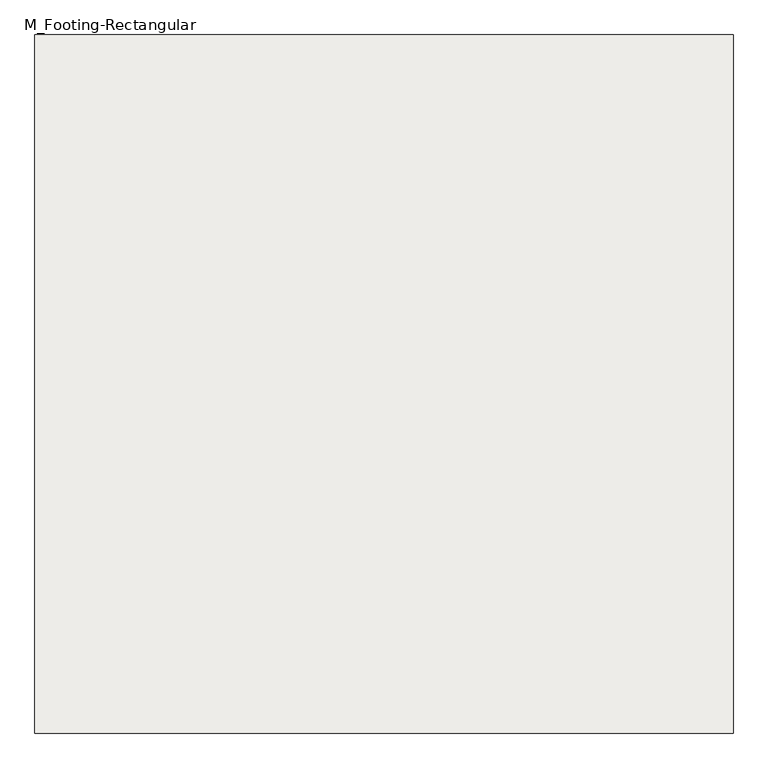
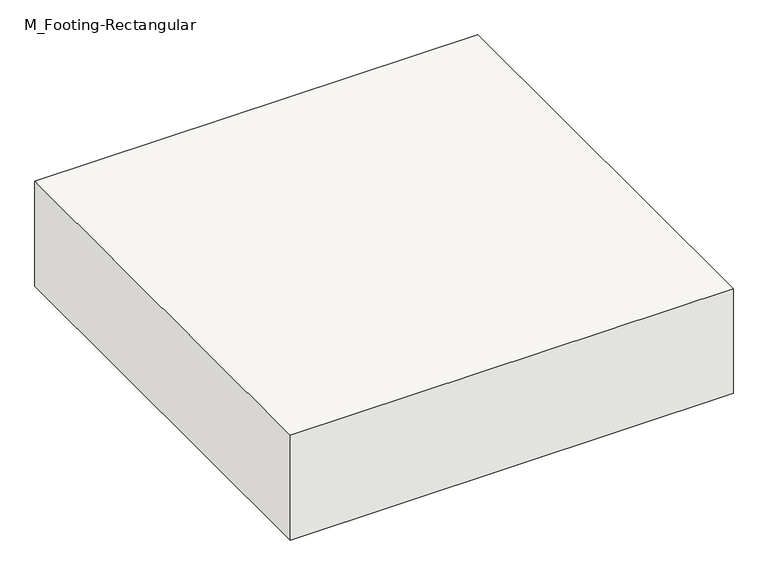
"""IFC4 building model written with IfcOpenShell, lengths in millimetres: slab geometry, M_Footing-Rectangular."""

from ifc_helpers import new_model, si_unit, frame, origin, place, context, project, spatial, polyline, outline, extrude, source, transform, mapped, element, save


def m_footing_rectangular_e5d4dde8(model_context):
    return source(origin(), model_context, "Body", "SweptSolid", [
        extrude(outline(polyline([(900.0, 900.0), (900.0, -900.0), (-900.0, -900.0), (-900.0, 900.0), (900.0, 900.0)])), frame((0.0, 0.0, -450.0), z_axis=(0.0, 0.0, 1.0), x_axis=(1.0, 0.0, 0.0)), (0.0, 0.0, 1.0), 450.0),
    ])


if __name__ == "__main__":
    model = new_model("IFC4")
    model_context = context("Model", 3, world=origin())
    ifc_project = project(units=[si_unit("LENGTHUNIT", "METRE", prefix="MILLI")], contexts=[model_context])
    site = spatial("IfcSite", under=ifc_project)
    building = spatial("IfcBuilding", under=site)
    placement = place(None, origin())
    m_footing_rectangular_shape = m_footing_rectangular_e5d4dde8(model_context)
    element("IfcSlab", 1, ObjectType="M_Footing-Rectangular", at=placement, inside=building, context=model_context, shape_type="MappedRepresentation", body=[
        mapped(m_footing_rectangular_shape, transform((0.0, 0.0, 0.0), x_axis=(1.0, 0.0, 0.0), y_axis=(0.0, 1.0, 0.0), z_axis=(0.0, 0.0, 1.0))),
    ])
    save(model, "model.ifc")

# Revit data of these elements
# Type "M_Footing-Rectangular"
#   Width = 1800 mm
#   Length = 1800 mm
#   Foundation Thickness = 450 mm
#   Structural Material [instance default] = Concrete, Cast-in-Place gray
#   Assembly Code = ""
# Element 1 (IfcSlab, "M_Footing-Rectangular")
#   Materials on its faces: "Concrete, Cast-in-Place gray"
# Materials
#   "Concrete, Cast-in-Place gray": class "Concrete", colour RGB 192 192 192, transparency 0, Description = "Cast-in-place concrete", Cost = 0
